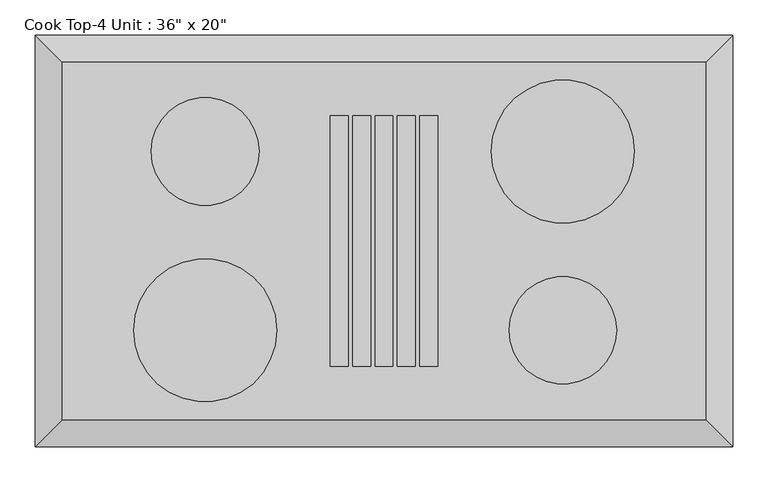
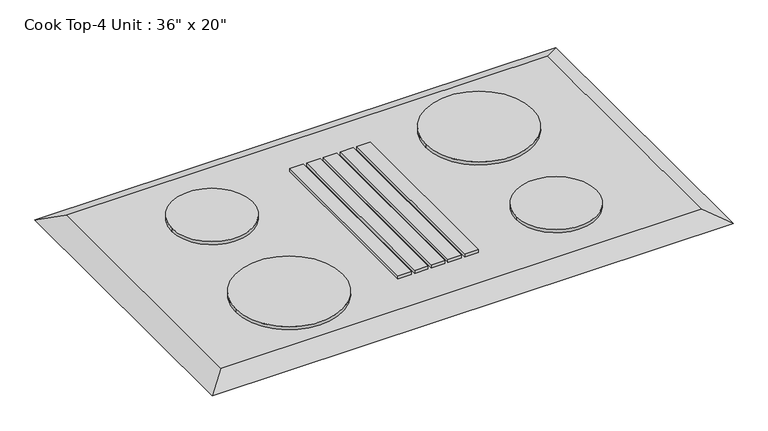
"""IFC4 building model written with IfcOpenShell, lengths in millimetres: proxy geometry."""

from ifc_helpers import new_model, si_unit, point, frame, frame_2d, origin, place, context, project, spatial, polyline, circle_curve, trimmed, segment, composite_curve, outline, extrude, faceted_brep, source, transform, mapped, element, save


def proxy_dd141328(model_context):
    return source(origin(), model_context, "Body", "SolidModel", [
        extrude(outline(composite_curve([segment(trimmed(circle_curve(frame_2d((-254.0, 127.0)), 76.5869489), [point((-177.4130511, 127.0))], [point((-330.5869489, 127.0))], False, "CARTESIAN"), True, "CONTINUOUS"), segment(trimmed(circle_curve(frame_2d((-254.0, 127.0)), 76.5869489), [point((-330.5869489, 127.0))], [point((-177.4130511, 127.0))], False, "CARTESIAN"), True, "CONTINUOUS")], self_intersect=False)), frame((0.0, 0.0, 806.45), z_axis=(0.0, 0.0, 1.0), x_axis=(1.0, 0.0, 0.0)), (0.0, 0.0, 1.0), 6.35),
        extrude(outline(composite_curve([segment(trimmed(circle_curve(frame_2d((254.0, 127.0)), 101.6), [point((355.6, 127.0))], [point((152.4, 127.0))], False, "CARTESIAN"), True, "CONTINUOUS"), segment(trimmed(circle_curve(frame_2d((254.0, 127.0)), 101.6), [point((152.4, 127.0))], [point((355.6, 127.0))], False, "CARTESIAN"), True, "CONTINUOUS")], self_intersect=False)), frame((0.0, 0.0, 806.45), z_axis=(0.0, 0.0, 1.0), x_axis=(1.0, 0.0, 0.0)), (0.0, 0.0, 1.0), 6.35),
        extrude(outline(composite_curve([segment(trimmed(circle_curve(frame_2d((254.0, -127.0)), 76.2), [point((330.2, -127.0))], [point((177.8, -127.0))], False, "CARTESIAN"), True, "CONTINUOUS"), segment(trimmed(circle_curve(frame_2d((254.0, -127.0)), 76.2), [point((177.8, -127.0))], [point((330.2, -127.0))], False, "CARTESIAN"), True, "CONTINUOUS")], self_intersect=False)), frame((0.0, 0.0, 806.45), z_axis=(0.0, 0.0, 1.0), x_axis=(1.0, 0.0, 0.0)), (0.0, 0.0, 1.0), 6.35),
        extrude(outline(polyline([(-50.8, 177.8), (-50.8, -177.8), (-76.2, -177.8), (-76.2, 177.8), (-50.8, 177.8)])), frame((0.0, 0.0, 806.45), z_axis=(0.0, 0.0, 1.0), x_axis=(1.0, 0.0, 0.0)), (0.0, 0.0, 1.0), 6.35),
        extrude(outline(polyline([(-19.05, 177.8), (-19.05, -177.8), (-44.45, -177.8), (-44.45, 177.8), (-19.05, 177.8)])), frame((0.0, 0.0, 806.45), z_axis=(0.0, 0.0, 1.0), x_axis=(1.0, 0.0, 0.0)), (0.0, 0.0, 1.0), 6.35),
        extrude(outline(polyline([(12.7, 177.8), (12.7, -177.8), (-12.7, -177.8), (-12.7, 177.8), (12.7, 177.8)])), frame((0.0, 0.0, 806.45), z_axis=(0.0, 0.0, 1.0), x_axis=(1.0, 0.0, 0.0)), (0.0, 0.0, 1.0), 6.35),
        extrude(outline(polyline([(44.45, 177.8), (44.45, -177.8), (19.05, -177.8), (19.05, 177.8), (44.45, 177.8)])), frame((0.0, 0.0, 806.45), z_axis=(0.0, 0.0, 1.0), x_axis=(1.0, 0.0, 0.0)), (0.0, 0.0, 1.0), 6.35),
        extrude(outline(polyline([(76.2, 177.8), (76.2, -177.8), (50.8, -177.8), (50.8, 177.8), (76.2, 177.8)])), frame((0.0, 0.0, 806.45), z_axis=(0.0, 0.0, 1.0), x_axis=(1.0, 0.0, 0.0)), (0.0, 0.0, 1.0), 6.35),
        faceted_brep([(457.2, 254.0, 806.45), (-457.2, 254.0, 806.45), (-457.2, -254.0, 806.45), (457.2, -254.0, 806.45), (495.3, 292.1, 787.4), (495.3, -292.1, 787.4), (-495.3, -292.1, 787.4), (-495.3, 292.1, 787.4)], [[[0, 1, 2, 3]], [[4, 5, 6, 7]], [[4, 7, 1, 0]], [[7, 6, 2, 1]], [[6, 5, 3, 2]], [[5, 4, 0, 3]]]),
        extrude(outline(composite_curve([segment(trimmed(circle_curve(frame_2d((-254.0, -127.0)), 101.6), [point((-152.4, -127.0))], [point((-355.6, -127.0))], False, "CARTESIAN"), True, "CONTINUOUS"), segment(trimmed(circle_curve(frame_2d((-254.0, -127.0)), 101.6), [point((-355.6, -127.0))], [point((-152.4, -127.0))], False, "CARTESIAN"), True, "CONTINUOUS")], self_intersect=False)), frame((0.0, 0.0, 806.45), z_axis=(0.0, 0.0, 1.0), x_axis=(1.0, 0.0, 0.0)), (0.0, 0.0, 1.0), 6.35),
    ])


if __name__ == "__main__":
    model = new_model("IFC4")
    model_context = context("Model", 3, world=origin())
    ifc_project = project(units=[si_unit("LENGTHUNIT", "METRE", prefix="MILLI")], contexts=[model_context])
    site = spatial("IfcSite", under=ifc_project)
    building = spatial("IfcBuilding", under=site)
    placement = place(None, origin())
    proxy_shape = proxy_dd141328(model_context)
    element("IfcBuildingElementProxy", 1, Name="Cook Top-4 Unit : 36\" x 20\"", ObjectType="Cook Top-4 Unit : 36\" x 20\"", at=placement, inside=building, context=model_context, shape_type="MappedRepresentation", body=[
        mapped(proxy_shape, transform((0.0, 0.0, 0.0), x_axis=(1.0, 0.0, 0.0), y_axis=(0.0, 1.0, 0.0), z_axis=(0.0, 0.0, 1.0))),
    ])
    save(model, "model.ifc")

# Revit data of these elements
# Type "Cook Top-4 Unit : 36\" x 20\""
#   Assembly Code = "E1090400"
#   Depth = 1' - 8"
#   Width = 3' - 0"
#   Burner Material = Steel, Chrome Plated
#   Cooktop Material = Steel, Polished
#   Default Elevation = 0
# Element 1 (IfcBuildingElementProxy, "Cook Top-4 Unit : 36\" x 20\"")
#   Materials on its faces: "Steel, Chrome Plated", "Steel, Polished"
# Materials
#   "Steel, Chrome Plated": class "Metal", colour RGB 17 17 17, transparency 0, Description = "Chromiuim plated steel", Cost = 0
#   "Steel, Polished": class "Metal", colour RGB 57 57 57, transparency 0, Description = "Polished steel", Cost = 0
